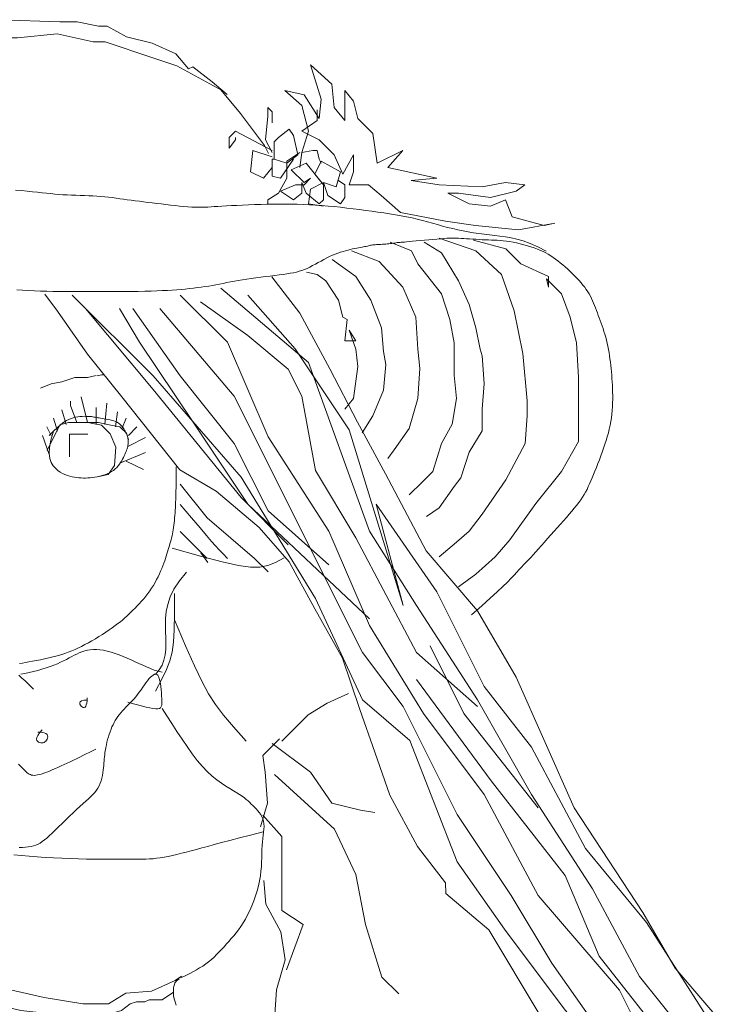
# Model space of a CAD drawing. Units: inches. Extents: x -17 to 1735, y -531 to 60.
# Tile 23 of 27: x 1734.803049 to 1734.807124, y -150.210609 to -150.204906. Entities that reach past the tile are written whole.
import ezdxf

# ---------------------------------------------------------------- set-up
doc = ezdxf.new("R2010")
doc.units = ezdxf.units.IN
doc.header["$MEASUREMENT"] = 0
doc.layers.add('A-FURN', color=242, linetype='Continuous', lineweight=18, true_color=0xcd2027)

# ---------------------------------------------------------------- blocks, each defined once
blk = doc.blocks.new('childrens_room_2')
for points in [[(73.37348, 54.43161), (73.37727, 54.43602), (73.37979, 54.43791), (73.38263, 54.44011), (73.38389, 54.442), (73.38704, 54.44358), (73.39051, 54.44452), (73.39429, 54.44578), (73.40375, 54.4483), (73.40753, 54.44862), (73.41132, 54.44893), (73.41447, 54.44893), (73.4233, 54.44862), (73.42582, 54.44862), (73.42898, 54.44799), (73.43024, 54.44799), (73.43307, 54.44641), (73.43686, 54.44547), (73.44033, 54.44389), (73.44222, 54.44169), (73.44285, 54.442), (73.44569, 54.4398), (73.44789, 54.43791)], [(73.3678, 54.42399), (73.37366, 54.43219), (73.3807, 54.43687), (73.38421, 54.43863), (73.39066, 54.44156), (73.39711, 54.4439), (73.40239, 54.44565), (73.40708, 54.44624), (73.41177, 54.44624), (73.41705, 54.44624), (73.42291, 54.44683), (73.42819, 54.44565), (73.42994, 54.44565), (73.43698, 54.44331), (73.4405, 54.44214), (73.44695, 54.43863), (73.44988, 54.43512), (73.4534, 54.43043), (73.45398, 54.42926)], [(73.45891, 54.42938), (73.45986, 54.43253), (73.45891, 54.4363), (73.45639, 54.43851), (73.45923, 54.43788), (73.46143, 54.43441), (73.46175, 54.43725), (73.46017, 54.44229), (73.46332, 54.43945), (73.46364, 54.43599), (73.46522, 54.4341), (73.46522, 54.43851), (73.46648, 54.43693), (73.46711, 54.43441), (73.46931, 54.43221), (73.46995, 54.4278), (73.47373, 54.42969), (73.47152, 54.42717), (73.47877, 54.4256), (73.47499, 54.42528), (73.47909, 54.42465), (73.4854, 54.42434), (73.48886, 54.42497), (73.4917, 54.42465), (73.49044, 54.42371), (73.48666, 54.42276), (73.48193, 54.42339), (73.48035, 54.42339), (73.4835, 54.42182), (73.48666, 54.4215), (73.48886, 54.42245), (73.48981, 54.41993), (73.49454, 54.41867), (73.49612, 54.41898), (73.49076, 54.41804), (73.48445, 54.41867), (73.48004, 54.4193), (73.47341, 54.42056), (73.47058, 54.42308), (73.46868, 54.42465), (73.46585, 54.42465), (73.46648, 54.42654), (73.46648, 54.42906), (73.4649, 54.42623), (73.46364, 54.42906), (73.46143, 54.43127), (73.45891, 54.43253), (73.46112, 54.4341), (73.46112, 54.43567)], [(73.4545, 54.42938), (73.45355, 54.43127), (73.45387, 54.43473), (73.45387, 54.43599), (73.4545, 54.43536), (73.4545, 54.43378)], [(73.4545, 54.42969), (73.44914, 54.43253), (73.44819, 54.43158), (73.44819, 54.43001), (73.44914, 54.43127), (73.44914, 54.43158)], [(73.45481, 54.42843), (73.45481, 54.43095), (73.45544, 54.43158), (73.45702, 54.43284), (73.45765, 54.4319), (73.45828, 54.42906), (73.4567, 54.4278), (73.45481, 54.42843), (73.4545, 54.42843), (73.4545, 54.42591), (73.45576, 54.4256), (73.45765, 54.42843)], [(73.4545, 54.42875), (73.45166, 54.42969), (73.45134, 54.42654), (73.45323, 54.4256), (73.4545, 54.42717)], [(73.45859, 54.42938), (73.4567, 54.42812), (73.4567, 54.4256), (73.45544, 54.42339), (73.45387, 54.42245), (73.45387, 54.42182)], [(73.45859, 54.42717), (73.45891, 54.42938), (73.46049, 54.42969), (73.46112, 54.42969), (73.46143, 54.42843), (73.46175, 54.4278)], [(73.46206, 54.4215), (73.45986, 54.42182), (73.46017, 54.42402), (73.46206, 54.42497), (73.46395, 54.42434), (73.46459, 54.42654), (73.46175, 54.42812), (73.4608, 54.42623), (73.46206, 54.42465), (73.45954, 54.4278), (73.45733, 54.42686), (73.45923, 54.42497), (73.46017, 54.4256), (73.45923, 54.42465), (73.45796, 54.42465), (73.45576, 54.42371), (73.45765, 54.42245), (73.45891, 54.42339), (73.45891, 54.42497), (73.45954, 54.42339), (73.46143, 54.42182), (73.46206, 54.42245), (73.46206, 54.42402), (73.46206, 54.42497), (73.46269, 54.42308), (73.46459, 54.42182), (73.46522, 54.42276), (73.46522, 54.42465), (73.46427, 54.42528)], [(73.41677, 54.42386), (73.41766, 54.42379), (73.4185, 54.42371), (73.41928, 54.42363), (73.42, 54.42355), (73.42068, 54.42348), (73.42132, 54.42341), (73.42194, 54.42334), (73.42255, 54.42328), (73.42315, 54.42323), (73.42375, 54.42318), (73.42437, 54.42315), (73.425, 54.42312), (73.42563, 54.4231), (73.42627, 54.42308), (73.4269, 54.42306), (73.42753, 54.42304), (73.42815, 54.42301), (73.42875, 54.42297), (73.42933, 54.42293), (73.4299, 54.42288), (73.43045, 54.42282), (73.431, 54.42275), (73.43155, 54.42268), (73.43209, 54.4226), (73.43265, 54.42253), (73.43321, 54.42245), (73.43379, 54.42237), (73.43438, 54.42229), (73.43499, 54.42221), (73.43561, 54.42213), (73.43624, 54.42205), (73.43689, 54.42198), (73.43754, 54.4219), (73.43821, 54.42182), (73.43888, 54.42174), (73.43956, 54.42166), (73.44023, 54.42159), (73.44089, 54.42152), (73.44152, 54.42146), (73.44214, 54.42141), (73.44271, 54.42137), (73.44325, 54.42135), (73.44374, 54.42133), (73.4442, 54.42133), (73.44464, 54.42135), (73.44508, 54.42137), (73.44553, 54.42139), (73.44601, 54.42143), (73.44655, 54.42146), (73.44714, 54.4215), (73.44781, 54.42154), (73.44854, 54.42158), (73.44934, 54.42162), (73.45017, 54.42165), (73.45105, 54.42169), (73.45194, 54.42172), (73.45285, 54.42174), (73.45376, 54.42177), (73.45466, 54.42178), (73.45556, 54.42179), (73.45645, 54.4218), (73.45733, 54.42179), (73.45822, 54.42178), (73.45911, 54.42175), (73.46, 54.42171), (73.46091, 54.42166), (73.46182, 54.42159), (73.46274, 54.42152), (73.46366, 54.42143), (73.46459, 54.42133), (73.46551, 54.42122), (73.46643, 54.42111), (73.46735, 54.42099), (73.46826, 54.42087), (73.46917, 54.42076), (73.47006, 54.42064), (73.47093, 54.42051), (73.4718, 54.42038), (73.47265, 54.42024), (73.47348, 54.4201), (73.4743, 54.41994), (73.4751, 54.41977), (73.47587, 54.41959), (73.47664, 54.41939), (73.47739, 54.41919), (73.47813, 54.41898), (73.47887, 54.41878), (73.4796, 54.41858), (73.48034, 54.41838), (73.48109, 54.4182), (73.48184, 54.41803), (73.4826, 54.41787), (73.48337, 54.41773), (73.48414, 54.4176), (73.48492, 54.41748), (73.4857, 54.41737), (73.48648, 54.41727), (73.48726, 54.41717), (73.48804, 54.41709), (73.48884, 54.41698), (73.48966, 54.41685), (73.49054, 54.41665), (73.49147, 54.41638), (73.4925, 54.41601), (73.49362, 54.41552), (73.49485, 54.41489)], [(73.41695, 54.4092), (73.41781, 54.40914), (73.41868, 54.40909), (73.41957, 54.40904), (73.42046, 54.40901), (73.42136, 54.40898), (73.42227, 54.40896), (73.4232, 54.40895), (73.42415, 54.40894), (73.42513, 54.40894), (73.42614, 54.40894), (73.42719, 54.40894), (73.42827, 54.40894), (73.42938, 54.40894), (73.4305, 54.40894), (73.43162, 54.40894), (73.43272, 54.40895), (73.43379, 54.40896), (73.43483, 54.40897), (73.43581, 54.40899), (73.43672, 54.40901), (73.43757, 54.40904), (73.43836, 54.40907), (73.43911, 54.40911), (73.43981, 54.40915), (73.44048, 54.4092), (73.44113, 54.40925), (73.44174, 54.40931), (73.44235, 54.40937), (73.44294, 54.40943), (73.44352, 54.40951), (73.44408, 54.40958), (73.44464, 54.40966), (73.44519, 54.40975), (73.44573, 54.40984), (73.44626, 54.40994), (73.44679, 54.41004), (73.44732, 54.41014), (73.44786, 54.41025), (73.44841, 54.41036), (73.44897, 54.41046), (73.44954, 54.41057), (73.45015, 54.41067), (73.45078, 54.41078), (73.45145, 54.41087), (73.45214, 54.41096), (73.45284, 54.41105), (73.45354, 54.41114), (73.45423, 54.41122), (73.45491, 54.4113), (73.45555, 54.41138), (73.45614, 54.41146), (73.45669, 54.41154), (73.45719, 54.41162), (73.45765, 54.41171), (73.45808, 54.41181), (73.45849, 54.41192), (73.45888, 54.41204), (73.45927, 54.41218), (73.45966, 54.41235), (73.46006, 54.41254), (73.46047, 54.41275), (73.46088, 54.41297), (73.4613, 54.4132), (73.46172, 54.41343), (73.46214, 54.41366), (73.46256, 54.41388), (73.46297, 54.41408), (73.46339, 54.41427), (73.46379, 54.41444), (73.46419, 54.41459), (73.46458, 54.41472), (73.46496, 54.41485), (73.46532, 54.41495), (73.46568, 54.41505), (73.46602, 54.41513), (73.46635, 54.41521), (73.46666, 54.41527), (73.46696, 54.41533), (73.46724, 54.41538), (73.4675, 54.41543), (73.46774, 54.41547), (73.46797, 54.41551), (73.46818, 54.41555), (73.46837, 54.41559), (73.46854, 54.41563), (73.4687, 54.41567), (73.46885, 54.4157), (73.46901, 54.41574), (73.46916, 54.41577), (73.46932, 54.41579), (73.46949, 54.41581), (73.46968, 54.41583), (73.46987, 54.41584), (73.47008, 54.41586), (73.4703, 54.41587), (73.47052, 54.41588), (73.47075, 54.41589), (73.47099, 54.4159), (73.47123, 54.41592), (73.47146, 54.41594), (73.47169, 54.41597), (73.47192, 54.41599), (73.47214, 54.41602), (73.47236, 54.41605), (73.47256, 54.41608), (73.47274, 54.41611), (73.47291, 54.41613), (73.47306, 54.41615), (73.4732, 54.41616), (73.47335, 54.41617), (73.47352, 54.41619), (73.47373, 54.4162), (73.47399, 54.41622), (73.4743, 54.41625), (73.47469, 54.41629), (73.47517, 54.41633), (73.47571, 54.41638), (73.4763, 54.41644), (73.47693, 54.4165), (73.47756, 54.41655), (73.47818, 54.41661), (73.47877, 54.41666), (73.47932, 54.41671), (73.4798, 54.41674), (73.48022, 54.41677), (73.4806, 54.41678), (73.48095, 54.41679), (73.48129, 54.41679), (73.48162, 54.41679), (73.48195, 54.41678), (73.48231, 54.41676), (73.4827, 54.41674), (73.48312, 54.41671), (73.48356, 54.41668), (73.48402, 54.41665), (73.48449, 54.41662), (73.48496, 54.4166), (73.48543, 54.41657), (73.48589, 54.41655), (73.48633, 54.41653), (73.48677, 54.41651), (73.4872, 54.4165), (73.48763, 54.41648), (73.48807, 54.41645), (73.48852, 54.41641), (73.48898, 54.41636), (73.48946, 54.41629), (73.48996, 54.4162), (73.49048, 54.41609), (73.49102, 54.41597), (73.49155, 54.41583), (73.49208, 54.41568), (73.49259, 54.41553), (73.49309, 54.41536), (73.49356, 54.41518), (73.494, 54.415), (73.4944, 54.41482), (73.49479, 54.41462), (73.49515, 54.41442), (73.49551, 54.4142), (73.49586, 54.41397), (73.4962, 54.41372), (73.49655, 54.41345), (73.49691, 54.41317), (73.49728, 54.41287), (73.49765, 54.41255), (73.49801, 54.41223), (73.49837, 54.41189), (73.49873, 54.41156), (73.49907, 54.41122), (73.49939, 54.41088), (73.4997, 54.41055), (73.49998, 54.41022), (73.50025, 54.40989), (73.5005, 54.40957), (73.50073, 54.40924), (73.50095, 54.40892), (73.50115, 54.40859), (73.50134, 54.40826), (73.50151, 54.40792), (73.50166, 54.40758), (73.50181, 54.40723), (73.50195, 54.40688), (73.50209, 54.40652), (73.50222, 54.40616), (73.50236, 54.40579), (73.50249, 54.40542), (73.50263, 54.40505), (73.50278, 54.40466), (73.50292, 54.40428), (73.50306, 54.40388), (73.5032, 54.40348), (73.50334, 54.40307), (73.50347, 54.40265), (73.5036, 54.40222), (73.50371, 54.40178), (73.50381, 54.40134), (73.50391, 54.40088), (73.504, 54.40042), (73.50408, 54.39996), (73.50415, 54.39949), (73.50422, 54.39902), (73.50428, 54.39855), (73.50434, 54.39807), (73.50439, 54.3976), (73.50443, 54.39712), (73.50448, 54.39664), (73.50451, 54.39616), (73.50454, 54.39567), (73.50457, 54.39517), (73.50459, 54.39466), (73.50461, 54.39415), (73.50462, 54.39362), (73.50462, 54.39309), (73.50461, 54.39255), (73.50459, 54.39201), (73.50456, 54.39146), (73.50451, 54.39091), (73.50444, 54.39036), (73.50435, 54.38981), (73.50424, 54.38926), (73.50412, 54.3887), (73.50398, 54.38815), (73.50382, 54.38759), (73.50365, 54.38703), (73.50347, 54.38647), (73.50328, 54.3859), (73.50308, 54.38533), (73.50287, 54.38475), (73.50266, 54.38418), (73.50244, 54.38362), (73.50222, 54.38307), (73.50201, 54.38254), (73.5018, 54.38203), (73.5016, 54.38154), (73.50141, 54.38108), (73.50122, 54.38065), (73.50103, 54.38024), (73.50084, 54.37984), (73.50063, 54.37945), (73.50042, 54.37906), (73.50018, 54.37868), (73.49992, 54.37829), (73.49963, 54.37789), (73.49931, 54.37748), (73.49896, 54.37706), (73.4986, 54.37662), (73.49821, 54.37617), (73.4978, 54.3757), (73.49737, 54.37522), (73.49692, 54.37472), (73.49646, 54.3742), (73.49599, 54.37367), (73.49552, 54.37313), (73.49505, 54.37259), (73.49459, 54.37207), (73.49414, 54.37156), (73.4937, 54.37108), (73.4933, 54.37063), (73.49292, 54.37021), (73.49256, 54.36983), (73.49222, 54.36946), (73.49188, 54.36911), (73.49155, 54.36877), (73.49122, 54.36841), (73.49087, 54.36805), (73.49051, 54.36766), (73.49012, 54.36724), (73.48967, 54.36676), (73.48912, 54.3662), (73.48845, 54.36554), (73.48763, 54.36475), (73.4866, 54.36381), (73.48535, 54.3627), (73.48384, 54.36139)], [(73.47186, 54.41618), (73.47501, 54.41492), (73.47595, 54.41303), (73.47942, 54.40862), (73.48068, 54.40484), (73.48131, 54.40138), (73.48131, 54.39666), (73.48163, 54.39319), (73.481, 54.38941), (73.47942, 54.38658), (73.47816, 54.38249), (73.47659, 54.38091), (73.47469, 54.37902)], [(73.4769, 54.41618), (73.47942, 54.41461), (73.48195, 54.41051), (73.48352, 54.40705), (73.48447, 54.40359), (73.4851, 54.40044), (73.48541, 54.39949), (73.48573, 54.3954), (73.48541, 54.39162), (73.48541, 54.38847), (73.48352, 54.38532), (73.48226, 54.38154), (73.48131, 54.38028), (73.47911, 54.37713), (73.47722, 54.37587)], [(73.47911, 54.41681), (73.48447, 54.41492), (73.48825, 54.41146), (73.49014, 54.4061), (73.4914, 54.39981), (73.49203, 54.39288), (73.49203, 54.39067), (73.49172, 54.38658), (73.48888, 54.38123), (73.48541, 54.37619), (73.48352, 54.37367), (73.48163, 54.37209), (73.47911, 54.36989)], [(73.48415, 54.4165), (73.48888, 54.41524), (73.49109, 54.41303), (73.49519, 54.41114), (73.49519, 54.40957), (73.49487, 54.41083), (73.49708, 54.40862), (73.49834, 54.40516), (73.49929, 54.40138), (73.4996, 54.39634), (73.4996, 54.39193), (73.4996, 54.3869), (73.49708, 54.38249), (73.4933, 54.37776), (73.48951, 54.37241), (73.48731, 54.36989), (73.48447, 54.36737), (73.48195, 54.36548)], [(73.46618, 54.41492), (73.47028, 54.41335), (73.47375, 54.40957), (73.47564, 54.40516), (73.47595, 54.40044), (73.47627, 54.3976), (73.47595, 54.39319), (73.47469, 54.38878), (73.47249, 54.38564), (73.47154, 54.38438)], [(73.46334, 54.41366), (73.46681, 54.41114), (73.46902, 54.40768), (73.47059, 54.40359), (73.47091, 54.40012), (73.47123, 54.39823), (73.47091, 54.39445), (73.46933, 54.39067), (73.46776, 54.38815)], [(73.45956, 54.41177), (73.46114, 54.41146), (73.4624, 54.41051), (73.46429, 54.40768), (73.46492, 54.40516), (73.46555, 54.40484), (73.46523, 54.4017), (73.46681, 54.4017), (73.46586, 54.40327), (73.46681, 54.40044), (73.46713, 54.39792), (73.4665, 54.39319), (73.46523, 54.39162)], [(73.45448, 54.41111), (73.45858, 54.40576), (73.46299, 54.39757), (73.46709, 54.3897), (73.47119, 54.38214), (73.47718, 54.3708), (73.48475, 54.36198), (73.49042, 54.35222), (73.49894, 54.33301), (73.50907, 54.3176), (73.5138, 54.30941), (73.52137, 54.3006), (73.52894, 54.29052), (73.53745, 54.28044), (73.54596, 54.26974), (73.55353, 54.26029), (73.56456, 54.24769), (73.56734, 54.24595)], [(73.44696, 54.40942), (73.45988, 54.3985), (73.46883, 54.37369), (73.47578, 54.36277), (73.48473, 54.34887), (73.49268, 54.33497), (73.50163, 54.32108), (73.50858, 54.30817), (73.52051, 54.29328), (73.53144, 54.28137), (73.54138, 54.27244), (73.54734, 54.26052), (73.56316, 54.2436)], [(73.42106, 54.40855), (73.42295, 54.40603), (73.42737, 54.39974), (73.43241, 54.39344), (73.44093, 54.38273), (73.44629, 54.37958), (73.45259, 54.37423), (73.45701, 54.36919), (73.46079, 54.36226), (73.46489, 54.35502), (73.46741, 54.34746), (73.46962, 54.34116), (73.47183, 54.33487), (73.47592, 54.32731), (73.48002, 54.32196), (73.48009, 54.32041), (73.48639, 54.31506), (73.49396, 54.30246), (73.50216, 54.29239), (73.51603, 54.27885), (73.52738, 54.26405), (73.54189, 54.24704), (73.54565, 54.24155)], [(73.42509, 54.40843), (73.43702, 54.39652), (73.44994, 54.38163), (73.46088, 54.36376), (73.46783, 54.34887), (73.47479, 54.34291), (73.48175, 54.32505), (73.4887, 54.31512), (73.49765, 54.30321), (73.50461, 54.29527), (73.51355, 54.28435), (73.52448, 54.27442), (73.53343, 54.26549), (73.54138, 54.25358), (73.55157, 54.24155)], [(73.441, 54.40843), (73.44795, 54.40148), (73.45392, 54.38758), (73.46286, 54.37369), (73.46883, 54.35979), (73.47678, 54.34688), (73.48572, 54.33497), (73.49367, 54.32008), (73.5056, 54.30619), (73.51355, 54.2903), (73.5215, 54.28435), (73.53244, 54.27442), (73.53343, 54.27045), (73.54834, 54.25655), (73.55927, 54.24266), (73.5601, 54.24155)], [(73.44398, 54.40744), (73.45094, 54.40247), (73.4569, 54.39751), (73.45889, 54.39354), (73.46088, 54.38262), (73.46684, 54.37269), (73.47578, 54.35582), (73.48473, 54.34788)], [(73.45094, 54.40843), (73.45789, 54.40049), (73.46584, 54.38858), (73.4738, 54.36277), (73.46982, 54.37766), (73.47877, 54.36475), (73.48572, 54.35086), (73.49268, 54.34192), (73.50063, 54.32703), (73.50958, 54.31611), (73.51852, 54.30222), (73.53244, 54.28336), (73.54436, 54.26946), (73.55629, 54.25556), (73.56679, 54.24595)], [(73.42708, 54.40644), (73.43702, 54.39453), (73.44994, 54.37865), (73.4569, 54.3717)], [(73.43205, 54.40644), (73.43503, 54.40148), (73.44298, 54.38957), (73.45094, 54.37766), (73.46883, 54.36078)], [(73.43404, 54.40644), (73.441, 54.39652), (73.44895, 54.38659), (73.45392, 54.37666), (73.46286, 54.36872)], [(73.43802, 54.40644), (73.44895, 54.39354), (73.46783, 54.35582), (73.4738, 54.34788), (73.48175, 54.332), (73.4897, 54.32008), (73.49566, 54.31016), (73.50262, 54.30023), (73.51057, 54.2903), (73.5215, 54.27839), (73.52945, 54.26847), (73.53741, 54.26052), (73.54238, 54.25655), (73.54933, 54.24663), (73.55079, 54.24155)], [(73.42044, 54.39471), (73.42202, 54.39534), (73.4236, 54.39565), (73.42549, 54.39628), (73.42738, 54.39628), (73.42864, 54.3966)], [(73.42877, 54.39654), (73.42942, 54.39671), (73.42974, 54.39671)], [(73.4258, 54.38967), (73.42486, 54.39219), (73.42486, 54.39282)], [(73.42738, 54.38967), (73.42643, 54.39345)], [(73.42423, 54.38936), (73.4236, 54.39156)], [(73.42864, 54.38936), (73.42864, 54.39187)], [(73.4299, 54.38936), (73.43022, 54.3925)], [(73.42235, 54.38841), (73.42197, 54.3871), (73.42178, 54.38601), (73.42174, 54.38511), (73.42183, 54.38438), (73.42203, 54.38379), (73.4223, 54.38331), (73.42263, 54.38294), (73.42298, 54.38263), (73.42333, 54.38238), (73.42368, 54.38217), (73.42404, 54.38201), (73.42439, 54.38187), (73.42474, 54.38177), (73.42508, 54.38169), (73.42542, 54.38163), (73.42576, 54.38158), (73.42609, 54.38155), (73.42642, 54.38153), (73.42675, 54.38151), (73.42708, 54.38151), (73.42741, 54.38152), (73.42775, 54.38155), (73.42809, 54.38158), (73.42844, 54.38164), (73.4288, 54.3817), (73.42916, 54.38178), (73.42953, 54.38188), (73.42989, 54.382), (73.43023, 54.38213), (73.43057, 54.38228), (73.43088, 54.38245), (73.43117, 54.38263), (73.43143, 54.38284), (73.43167, 54.38306), (73.43188, 54.3833), (73.43207, 54.38354), (73.43223, 54.38379), (73.43239, 54.38404), (73.43252, 54.38428), (73.43264, 54.38452), (73.43276, 54.38475), (73.43286, 54.38498), (73.43296, 54.38519), (73.43304, 54.3854), (73.43311, 54.38559), (73.43318, 54.38578), (73.43323, 54.38597), (73.43328, 54.38615), (73.43331, 54.38632), (73.43333, 54.38649), (73.43335, 54.38666), (73.43335, 54.38683), (73.43335, 54.38699), (73.43333, 54.38715), (73.43331, 54.3873), (73.43328, 54.38746), (73.43323, 54.38762), (73.43318, 54.38778), (73.43312, 54.38793), (73.43305, 54.38809), (73.43297, 54.38825), (73.43288, 54.38841), (73.43279, 54.38856), (73.4327, 54.38872), (73.4326, 54.38888), (73.43249, 54.38903), (73.43237, 54.38919), (73.43223, 54.38933), (73.43208, 54.38947), (73.43191, 54.3896), (73.43171, 54.38972), (73.43149, 54.38982), (73.43124, 54.38991), (73.43097, 54.38999), (73.43068, 54.39006), (73.43039, 54.39012), (73.43009, 54.39017), (73.4298, 54.39021), (73.42953, 54.39026), (73.42928, 54.3903), (73.42906, 54.39034), (73.42886, 54.39037), (73.42867, 54.39041), (73.42849, 54.39045), (73.42831, 54.39048), (73.42813, 54.39051), (73.42793, 54.39054), (73.42771, 54.39056), (73.42745, 54.39058), (73.42718, 54.39058), (73.42688, 54.39059), (73.42657, 54.39057), (73.42625, 54.39055), (73.42592, 54.39051), (73.42559, 54.39045), (73.42526, 54.39037), (73.42494, 54.39027), (73.42461, 54.39013), (73.42426, 54.38995), (73.42387, 54.3897), (73.42344, 54.38937), (73.42294, 54.38895), (73.42237, 54.38842), (73.42171, 54.38778)], [(73.42296, 54.38841), (73.42233, 54.3903)], [(73.43148, 54.38904), (73.43179, 54.39124)], [(73.43242, 54.38873), (73.43305, 54.3903)], [(73.42202, 54.38778), (73.42139, 54.38904)], [(73.4214, 54.38557), (73.42329, 54.38935), (73.42455, 54.38967), (73.42707, 54.38967), (73.42897, 54.38967), (73.43054, 54.38935), (73.43212, 54.38904), (73.43307, 54.38809), (73.43338, 54.38715)], [(73.42764, 54.38961), (73.42942, 54.38929), (73.43071, 54.388), (73.43151, 54.38607), (73.43135, 54.38333), (73.43038, 54.38204), (73.42909, 54.38172)], [(73.43337, 54.38778), (73.43463, 54.38904)], [(73.4217, 54.38495), (73.42076, 54.38778)], [(73.4274, 54.38797), (73.4247, 54.38797), (73.4247, 54.3846), (73.4247, 54.3846)], [(73.43337, 54.38621), (73.43589, 54.38747)], [(73.43211, 54.38369), (73.43589, 54.38526)], [(73.41736, 54.35423), (73.41779, 54.35429), (73.41824, 54.35437), (73.41874, 54.35445), (73.41927, 54.35455), (73.41984, 54.35466), (73.42043, 54.35478), (73.42104, 54.35491), (73.42166, 54.35505), (73.42227, 54.3552), (73.42287, 54.35536), (73.42344, 54.35552), (73.424, 54.3557), (73.42452, 54.35588), (73.42503, 54.35608), (73.42552, 54.35629), (73.42601, 54.35651), (73.42649, 54.35674), (73.42698, 54.357), (73.42748, 54.35727), (73.42799, 54.35756), (73.42851, 54.35787), (73.42903, 54.35819), (73.42955, 54.35851), (73.43005, 54.35884), (73.43054, 54.35917), (73.431, 54.35949), (73.43143, 54.3598), (73.43183, 54.36009), (73.43219, 54.36037), (73.43253, 54.36065), (73.43285, 54.36092), (73.43315, 54.3612), (73.43345, 54.36147), (73.43374, 54.36176), (73.43404, 54.36205), (73.43435, 54.36236), (73.43466, 54.36269), (73.43498, 54.36302), (73.4353, 54.36338), (73.43562, 54.36374), (73.43593, 54.36411), (73.43623, 54.3645), (73.43652, 54.3649), (73.43679, 54.36531), (73.43705, 54.36572), (73.4373, 54.36614), (73.43753, 54.36656), (73.43774, 54.36698), (73.43794, 54.3674), (73.43812, 54.36781), (73.43829, 54.3682), (73.43845, 54.36859), (73.43859, 54.36896), (73.43872, 54.36933), (73.43883, 54.36968), (73.43894, 54.37002), (73.43904, 54.37035), (73.43914, 54.37066), (73.43923, 54.37097), (73.43932, 54.37127), (73.43941, 54.37156), (73.43949, 54.37184), (73.43957, 54.37213), (73.43965, 54.37241), (73.43972, 54.37269), (73.43979, 54.37298), (73.43985, 54.37328), (73.43991, 54.37359), (73.43996, 54.37391), (73.44001, 54.37423), (73.44006, 54.37457), (73.4401, 54.37491), (73.44014, 54.37526), (73.44017, 54.37563), (73.4402, 54.37599), (73.44023, 54.37637), (73.44026, 54.37675), (73.44028, 54.37715), (73.4403, 54.37754), (73.44032, 54.37795), (73.44034, 54.37836), (73.44035, 54.37878), (73.44036, 54.3792), (73.44037, 54.37964), (73.44038, 54.38008), (73.44038, 54.38053), (73.44039, 54.38101), (73.44039, 54.38151), (73.44039, 54.38203), (73.44039, 54.38258), (73.44039, 54.38317)], [(73.43305, 54.384), (73.43558, 54.38274)], [(73.441, 54.38061), (73.44498, 54.37565), (73.45194, 54.36969), (73.45392, 54.36771)], [(73.441, 54.37763), (73.44265, 54.37566), (73.44391, 54.37416), (73.44486, 54.37303), (73.4456, 54.37217), (73.4462, 54.37151), (73.44673, 54.37093), (73.4473, 54.37036), (73.44796, 54.36969)], [(73.441, 54.37366), (73.44498, 54.36969)], [(73.4398, 54.37119), (73.44398, 54.37003), (73.44717, 54.36919), (73.44955, 54.36865), (73.45134, 54.36838), (73.45271, 54.36838), (73.45387, 54.36862), (73.455, 54.3691), (73.4563, 54.36978)], [(73.44507, 54.36908), (73.44401, 54.37049)], [(73.44191, 54.36768), (73.44087, 54.3664), (73.44008, 54.36518), (73.43952, 54.36402), (73.43915, 54.36291), (73.43894, 54.36185), (73.43884, 54.36083), (73.43881, 54.35986), (73.43884, 54.35892), (73.43887, 54.35802), (73.43889, 54.35714), (73.43887, 54.35631), (73.43878, 54.3555), (73.43861, 54.35473), (73.43833, 54.35399), (73.43792, 54.35328), (73.43735, 54.35261)], [(73.42856, 54.34161), (73.42809, 54.34138), (73.42762, 54.34114), (73.42715, 54.34091), (73.42668, 54.34067), (73.42621, 54.34044), (73.42575, 54.34022), (73.42529, 54.33999), (73.42483, 54.33977), (73.42438, 54.33956), (73.42394, 54.33935), (73.4235, 54.33915), (73.42308, 54.33896), (73.42266, 54.33878), (73.42227, 54.33861), (73.42188, 54.33845), (73.42152, 54.3383), (73.42118, 54.33817), (73.42085, 54.33806), (73.42054, 54.33796), (73.42026, 54.33789), (73.41999, 54.33783), (73.41975, 54.33779), (73.41952, 54.33777), (73.41931, 54.33778), (73.41913, 54.33781), (73.41895, 54.33787), (73.41879, 54.33794), (73.41864, 54.33804), (73.41848, 54.33816), (73.41833, 54.3383), (73.41817, 54.33845), (73.418, 54.33862), (73.41782, 54.3388), (73.41762, 54.339), (73.41742, 54.33921), (73.41721, 54.33943)], [(73.44015, 54.36453), (73.44015, 54.36151), (73.44011, 54.35918), (73.44, 54.35736), (73.4398, 54.3559), (73.43947, 54.35461), (73.43897, 54.35334), (73.43827, 54.35191), (73.43735, 54.35016)], [(73.41724, 54.35251), (73.41767, 54.35212), (73.41817, 54.35165), (73.41875, 54.35109), (73.41942, 54.35043)], [(73.44015, 54.36067), (73.44179, 54.35684), (73.44308, 54.35389), (73.44416, 54.3516), (73.44515, 54.34976), (73.44618, 54.34817), (73.44736, 54.34662), (73.44882, 54.3449), (73.45068, 54.3428)], [(73.47777, 54.35681), (73.48274, 54.34688), (73.49367, 54.33299)], [(73.41753, 54.35263), (73.41813, 54.35276), (73.41876, 54.3529), (73.41939, 54.35305), (73.42003, 54.35321), (73.42066, 54.35339), (73.42127, 54.35357), (73.42186, 54.35377), (73.42241, 54.35397), (73.42292, 54.35418), (73.4234, 54.3544), (73.42384, 54.35461), (73.42425, 54.35483), (73.42465, 54.35504), (73.42503, 54.35524), (73.4254, 54.35544), (73.42578, 54.35562), (73.42615, 54.35579), (73.42654, 54.35594), (73.42694, 54.35607), (73.42735, 54.35618), (73.42777, 54.35625), (73.42822, 54.35629), (73.42869, 54.35629), (73.42919, 54.35625), (73.42972, 54.35617), (73.43027, 54.35605), (73.43084, 54.3559), (73.43142, 54.35571), (73.43201, 54.3555), (73.43261, 54.35527), (73.4332, 54.35502), (73.43379, 54.35476), (73.43437, 54.35449), (73.43493, 54.35422), (73.43549, 54.35396), (73.43605, 54.35371), (73.43661, 54.35347), (73.43718, 54.35326), (73.43775, 54.35309), (73.43834, 54.35295)], [(73.4173, 54.32715), (73.41778, 54.32717), (73.41823, 54.32719), (73.41865, 54.32724), (73.41905, 54.3273), (73.41942, 54.32739), (73.41976, 54.3275), (73.42008, 54.32764), (73.42039, 54.32781), (73.42071, 54.32802), (73.42103, 54.32826), (73.42137, 54.32855), (73.42174, 54.32889), (73.42215, 54.32928), (73.42261, 54.32972), (73.4231, 54.3302), (73.42362, 54.3307), (73.42416, 54.33123), (73.4247, 54.33175), (73.42524, 54.33227), (73.42576, 54.33276), (73.42625, 54.33321), (73.4267, 54.33362), (73.42712, 54.33399), (73.4275, 54.33433), (73.42784, 54.33465), (73.42815, 54.33496), (73.42842, 54.33526), (73.42866, 54.33557), (73.42888, 54.33589), (73.42906, 54.33624), (73.42922, 54.3366), (73.42935, 54.33698), (73.42946, 54.33737), (73.42954, 54.33776), (73.42962, 54.33814), (73.42967, 54.33852), (73.42972, 54.33888), (73.42975, 54.33923), (73.42978, 54.33956), (73.42981, 54.33988), (73.42983, 54.34019), (73.42986, 54.34051), (73.42989, 54.34083), (73.42993, 54.34116), (73.42998, 54.34151), (73.43005, 54.34187), (73.43013, 54.34225), (73.43022, 54.34264), (73.43032, 54.34303), (73.43044, 54.34342), (73.43056, 54.34381), (73.43069, 54.34419), (73.43082, 54.34455), (73.43096, 54.3449), (73.43111, 54.34522), (73.43127, 54.34554), (73.43143, 54.34584), (73.43161, 54.34613), (73.4318, 54.34641), (73.43201, 54.34669), (73.43224, 54.34696), (73.43249, 54.34724), (73.43275, 54.34752), (73.43302, 54.3478), (73.4333, 54.34809), (73.43359, 54.34838), (73.43388, 54.34868), (73.43417, 54.349), (73.43445, 54.34933), (73.43472, 54.34967), (73.43498, 54.35002), (73.43523, 54.35037), (73.43548, 54.35072), (73.43572, 54.35106), (73.43595, 54.35138), (73.43617, 54.35168), (73.43639, 54.35195), (73.43661, 54.35219), (73.43681, 54.35238), (73.43701, 54.35253), (73.4372, 54.35263), (73.43738, 54.35266), (73.43754, 54.35262), (73.43768, 54.35251), (73.43781, 54.35232), (73.43792, 54.35204), (73.43801, 54.35169), (73.43808, 54.35129), (73.43815, 54.35085), (73.43819, 54.35039), (73.43823, 54.34993), (73.43826, 54.34948), (73.43828, 54.34906), (73.4383, 54.3487), (73.4383, 54.34838), (73.43827, 54.34811), (73.43821, 54.34789), (73.4381, 54.34772), (73.43794, 54.34761), (73.4377, 54.34755), (73.43739, 54.34754), (73.43699, 54.34759), (73.43653, 54.34768), (73.43601, 54.3478), (73.43546, 54.34794), (73.43489, 54.3481), (73.43433, 54.34826), (73.43379, 54.34841), (73.43329, 54.34854)], [(73.47578, 54.35185), (73.48672, 54.33696), (73.49765, 54.32306), (73.50262, 54.31115), (73.51355, 54.29725), (73.5225, 54.28931), (73.53343, 54.27541), (73.5384, 54.26847), (73.54436, 54.26449), (73.54834, 54.26052)], [(73.45595, 54.3428), (73.45981, 54.34665), (73.46261, 54.3484), (73.46577, 54.34981)], [(73.4273, 54.34885), (73.4268, 54.34882), (73.42647, 54.34873), (73.42628, 54.34859), (73.42621, 54.34843), (73.42623, 54.34826), (73.42631, 54.34809), (73.42644, 54.34794), (73.42659, 54.34783), (73.42673, 54.34777), (73.42687, 54.34776), (73.42699, 54.34782), (73.42709, 54.34794), (73.42718, 54.34813), (73.42725, 54.3484), (73.42729, 54.34874), (73.4273, 54.34917)], [(73.43834, 54.34759), (73.43905, 54.34651), (73.43978, 54.34538), (73.44052, 54.34424), (73.44126, 54.34311), (73.44201, 54.342), (73.44276, 54.34095), (73.44351, 54.33997), (73.44425, 54.33909), (73.44498, 54.33832), (73.4457, 54.33766), (73.4464, 54.33709), (73.44707, 54.3366), (73.4477, 54.33618), (73.44829, 54.33582), (73.44883, 54.3355), (73.44932, 54.33521), (73.44974, 54.33494), (73.45011, 54.33469), (73.45043, 54.33445), (73.45072, 54.33422), (73.45098, 54.334), (73.45122, 54.33378), (73.45145, 54.33355), (73.45168, 54.33332), (73.45192, 54.33308), (73.45217, 54.33283), (73.4524, 54.33256), (73.45263, 54.33228), (73.45284, 54.33199), (73.45301, 54.33168), (73.45316, 54.33135), (73.45326, 54.33101), (73.45332, 54.33065), (73.45333, 54.33026), (73.45331, 54.32985), (73.45327, 54.32942), (73.45322, 54.32897), (73.45316, 54.32849), (73.4531, 54.32798), (73.45305, 54.32744), (73.45302, 54.32688), (73.453, 54.32628), (73.45298, 54.32566), (73.45296, 54.32502), (73.45293, 54.32435), (73.45288, 54.32367), (73.4528, 54.32297), (73.45268, 54.32224), (73.45252, 54.32151), (73.45232, 54.32077), (73.45209, 54.32003), (73.45183, 54.3193), (73.45154, 54.31859), (73.45123, 54.3179), (73.45091, 54.31724), (73.45058, 54.31663), (73.45024, 54.31606), (73.4499, 54.31554), (73.44956, 54.31505), (73.44921, 54.3146), (73.44886, 54.31416), (73.4485, 54.31375), (73.44815, 54.31335), (73.44779, 54.31296), (73.44744, 54.31256), (73.44708, 54.31217), (73.44672, 54.31179), (73.44635, 54.31141), (73.44597, 54.31104), (73.44558, 54.31068), (73.44517, 54.31034), (73.44475, 54.31002), (73.44431, 54.30971), (73.44385, 54.30943), (73.4434, 54.30916), (73.44295, 54.30891), (73.44251, 54.30869), (73.4421, 54.30848), (73.44172, 54.30829), (73.44138, 54.30813), (73.44109, 54.30798)], [(73.42068, 54.34445), (73.42028, 54.34401), (73.42003, 54.34364), (73.4199, 54.34334), (73.41987, 54.34309), (73.41992, 54.3429), (73.42003, 54.34275), (73.42017, 54.34265), (73.42034, 54.34258), (73.4205, 54.34255), (73.42066, 54.34255), (73.42082, 54.34257), (73.42097, 54.34262), (73.4211, 54.3427), (73.42122, 54.34281), (73.42133, 54.34293), (73.42141, 54.34308), (73.42148, 54.34325), (73.42151, 54.34342), (73.42149, 54.3436), (73.4214, 54.34376), (73.42123, 54.34391), (73.42096, 54.34403), (73.42057, 54.3441), (73.42005, 54.34413)], [(73.45559, 54.34315), (73.45314, 54.34069), (73.45349, 54.33824), (73.45384, 54.33368), (73.45279, 54.33018)], [(73.45454, 54.34245), (73.46016, 54.33824), (73.46331, 54.33368), (73.46753, 54.33263), (73.46963, 54.33228)], [(73.41654, 54.32608), (73.41763, 54.32597), (73.41877, 54.32587), (73.41994, 54.32578), (73.42114, 54.3257), (73.42236, 54.32563), (73.42359, 54.32558), (73.42481, 54.32553), (73.42603, 54.32549), (73.42722, 54.32546), (73.42838, 54.32544), (73.4295, 54.32543), (73.43057, 54.32542), (73.43157, 54.32542), (73.4325, 54.32542), (73.43335, 54.32542), (73.4341, 54.32542), (73.43478, 54.32542), (73.43539, 54.32543), (73.43596, 54.32544), (73.43649, 54.32547), (73.43701, 54.32551), (73.43753, 54.32557), (73.43806, 54.32564), (73.43863, 54.32573), (73.43922, 54.32585), (73.43984, 54.32598), (73.4405, 54.32613), (73.44118, 54.3263), (73.44189, 54.32648), (73.44263, 54.32667), (73.4434, 54.32687), (73.44419, 54.32709), (73.44505, 54.32732), (73.446, 54.32758), (73.44707, 54.32787), (73.44829, 54.32819), (73.4497, 54.32856), (73.45134, 54.32898), (73.45322, 54.32945)], [(73.45489, 54.33789), (73.46367, 54.32983), (73.46682, 54.32317), (73.46823, 54.31581), (73.47068, 54.3081), (73.47314, 54.30564)], [(73.45314, 54.33193), (73.45595, 54.32878), (73.45595, 54.31791)], [(73.36613, 54.32398), (73.37496, 54.31894), (73.37969, 54.31862), (73.38568, 54.3161), (73.39451, 54.31296), (73.40334, 54.30981), (73.41122, 54.30729), (73.42099, 54.30508), (73.42667, 54.30414), (73.43045, 54.30414), (73.43298, 54.30571), (73.43676, 54.30603), (73.44023, 54.3076), (73.44117, 54.30823)], [(73.45329, 54.3223), (73.4536, 54.31884), (73.45581, 54.31475), (73.45644, 54.31065), (73.45518, 54.30624), (73.45486, 54.30183)], [(73.36676, 54.32146), (73.37149, 54.31862), (73.37591, 54.31673), (73.37938, 54.31642), (73.3819, 54.31516), (73.38568, 54.31296), (73.38915, 54.31233), (73.39419, 54.31044), (73.39829, 54.30981), (73.40302, 54.30729), (73.40744, 54.30603), (73.41343, 54.30414), (73.41753, 54.30319), (73.42604, 54.30225), (73.43014, 54.30256), (73.43235, 54.30319), (73.43361, 54.30414), (73.43455, 54.30445), (73.4355, 54.30445), (73.43581, 54.30445), (73.43644, 54.30477), (73.43834, 54.30477), (73.43999, 54.30587)], [(73.45595, 54.31791), (73.4591, 54.31581), (73.45665, 54.30915)], [(73.44085, 54.30784), (73.44064, 54.3077), (73.44047, 54.30756), (73.44033, 54.30741), (73.44022, 54.30723), (73.44014, 54.30701), (73.44007, 54.30676), (73.44002, 54.30646), (73.43999, 54.30612), (73.43999, 54.30574), (73.44002, 54.30533), (73.4401, 54.3049), (73.44023, 54.30444), (73.44041, 54.30398)]]:
    blk.add_lwpolyline(points)

msp = doc.modelspace()

# ---------------------------------------------------------------- block references
at = {"layer": 'A-FURN', "xscale": 0.0393700787401575, "yscale": 0.0393700787401575, "zscale": 0.0393700787401575}
msp.add_blockref('childrens_room_2', (1731.9126009, -152.348565), dxfattribs=at)

doc.saveas('drawing.dxf')
